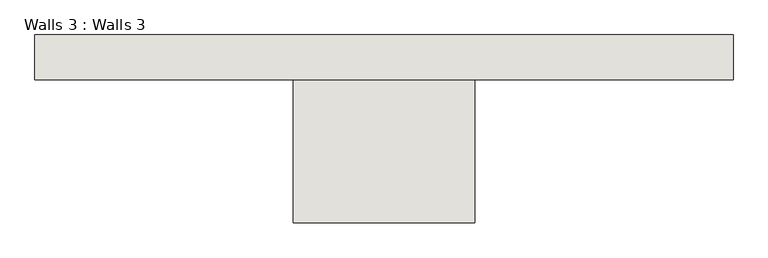
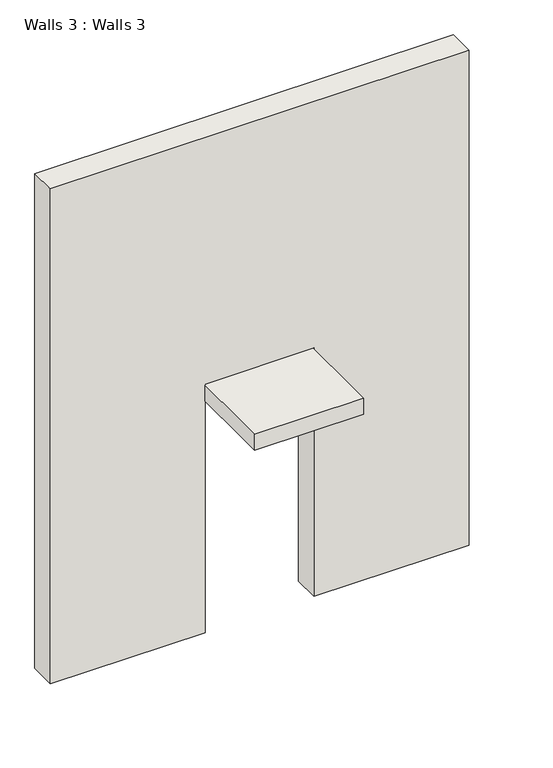
"""IFC4 building model written with IfcOpenShell, lengths in millimetres: wall geometry, Walls 3 : Walls 3."""

from ifc_helpers import new_model, si_unit, frame, origin, place, context, project, spatial, polyline, outline, extrude, source, transform, mapped, element, save


def walls_3_walls_3_bd47f883(model_context):
    return source(origin(), model_context, "Body", "SweptSolid", [
        extrude(outline(polyline([(924.5818298, -1637.0672508), (-27.9181702, -1637.0672508), (-27.9181702, -652.5387835), (924.5818298, -652.5387835), (924.5818298, -1637.0672508)])), frame((0.0, 0.0, 2139.4433014), z_axis=(0.0, 0.0, 1.0), x_axis=(1.0, 0.0, 0.0)), (0.0, 0.0, 1.0), 146.8011093),
        extrude(outline(polyline([(0.0, -27.9181702), (933.45, -27.9181702), (2296.0958758, -27.9181702), (2296.0958758, 924.5818298), (0.0, 924.5818298), (0.0, 2277.1318298), (609.6, 2277.1318298), (4572.0, 2277.1318298), (4572.0, -1380.4681702), (0.0, -1380.4681702), (0.0, -27.9181702)])), frame((0.0, -887.0605557, 0.0), z_axis=(0.0, 1.0, 0.0), x_axis=(0.0, 0.0, 1.0)), (0.0, 0.0, 1.0), 234.5217722),
    ])


if __name__ == "__main__":
    model = new_model("IFC4")
    model_context = context("Model", 3, world=origin())
    ifc_project = project(units=[si_unit("LENGTHUNIT", "METRE", prefix="MILLI")], contexts=[model_context])
    site = spatial("IfcSite", under=ifc_project)
    building = spatial("IfcBuilding", under=site)
    placement = place(None, origin())
    walls_3_walls_3_shape = walls_3_walls_3_bd47f883(model_context)
    element("IfcWall", 1, ObjectType="Walls 3 : Walls 3", at=placement, inside=building, context=model_context, shape_type="MappedRepresentation", body=[
        mapped(walls_3_walls_3_shape, transform((0.0, 0.0, 0.0), x_axis=(1.0, 0.0, 0.0), y_axis=(0.0, 1.0, 0.0), z_axis=(0.0, 0.0, 1.0))),
    ])
    save(model, "model.ifc")

# Revit data of these elements
# Element 1 (IfcWall, "Walls 3 : Walls 3")
#   Materials on its faces: "Default Wall"
# Materials
#   "Default Wall": colour RGB 128 128 128, transparency 0
